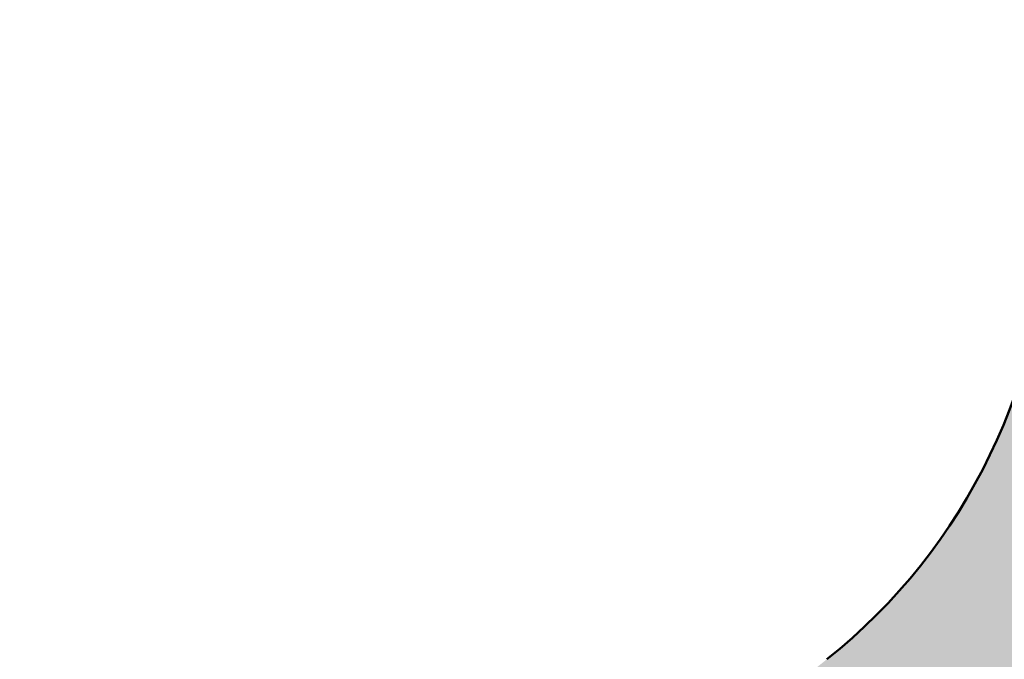
# Model space of a CAD drawing. Units: millimetres. Extents: x 0 to 2267, y 0 to 1823.
# Tile 21 of 256: x 1506 to 1590, y 1162 to 1217. Entities that reach past the tile are written whole.
import ezdxf

# ---------------------------------------------------------------- set-up
doc = ezdxf.new("R2010")
doc.units = ezdxf.units.MM
doc.header["$MEASUREMENT"] = 0
doc.layers.add('M-HATC', color=252, linetype='Continuous', lineweight=18)
doc.layers.add('M-OUTL', color=7, linetype='Continuous', lineweight=50)

msp = doc.modelspace()

# ---------------------------------------------------------------- hatches: boundary and pattern name
at = {"layer": 'M-HATC'}
h = msp.add_hatch(color=256, dxfattribs=at)
h.dxf.hatch_style = 1
h.paths.add_polyline_path([(2055.771, 1603.062), (1381.087, 1603.062), (1381.087, 1598.062), (2055.771, 1598.062)])
h.paths.add_polyline_path([(2055.771, 1598.062), (1381.087, 1598.062), (1381.087, 1593.062), (2055.771, 1593.062)])
h.paths.add_polyline_path([(2051.307, 1536.761), (1385.55, 1536.761), (1385.55, 1526.761), (1387.55, 1526.761), (1388.537, 1525.053), (1385.332, 1521.233), (1385.332, 1521.223), (2050.254, 1522.749), (2048.321, 1525.053), (2049.307, 1526.761), (2051.307, 1526.761)])
edge = h.paths.add_edge_path()
edge.add_arc((1847.535, 1379.149), 135, 222.60306, 222.89085, ccw=False)
edge.add_line((1748.166, 1287.766), (1683.092, 1287.766))
edge.add_arc((1583.724, 1379.149), 135, 317.10915, 317.39694, ccw=False)
edge.add_arc((1678.969, 1290.671), 5, 222.89085, 317.10915, ccw=False)
edge.add_arc((1774.213, 1379.149), 135, 222.60306, 222.89085, ccw=False)
edge.add_line((1674.845, 1287.766), (1609.771, 1287.766))
edge.add_arc((1510.403, 1379.149), 135, 317.10915, 317.39694, ccw=False)
edge.add_arc((1605.647, 1290.671), 5, 222.89085, 317.10915, ccw=False)
edge.add_arc((1700.892, 1379.149), 135, 222.60306, 222.89085, ccw=False)
edge.add_line((1601.524, 1287.766), (1536.45, 1287.766))
edge.add_arc((1437.081, 1379.149), 135, 317.10915, 317.39694, ccw=False)
edge.add_arc((1532.326, 1290.671), 5, 222.89085, 317.10915, ccw=False)
edge.add_arc((1627.571, 1379.149), 135, 222.60306, 222.89085, ccw=False)
edge.add_line((1528.203, 1287.766), (1505.929, 1287.766))
edge.add_spline(control_points=[(1505.929, 1287.766), (1504.262, 1287.766), (1504.262, 1282.766), (1505.929, 1282.766)], knot_values=[0, 0, 0, 0, 5, 5, 5, 5], degree=3, periodic=0)
edge.add_line((1505.929, 1282.766), (1930.929, 1282.766))
edge.add_spline(control_points=[(1930.929, 1282.766), (1932.596, 1282.766), (1932.596, 1287.766), (1930.929, 1287.766)], knot_values=[0, 0, 0, 0, 5, 5, 5, 5], degree=3, periodic=0)
edge.add_line((1930.929, 1287.766), (1903.056, 1287.766))
edge.add_arc((1803.688, 1379.149), 135, 317.10915, 317.39694, ccw=False)
edge.add_arc((1898.932, 1290.671), 5, 222.89085, 317.10915, ccw=False)
edge.add_arc((1994.177, 1379.149), 135, 222.60306, 222.89085, ccw=False)
edge.add_line((1894.809, 1287.766), (1829.735, 1287.766))
edge.add_arc((1730.366, 1379.149), 135, 317.10915, 317.39694, ccw=False)
edge.add_arc((1825.611, 1290.671), 5, 222.89085, 317.10915, ccw=False)
edge.add_arc((1920.856, 1379.149), 135, 222.60306, 222.89085, ccw=False)
edge.add_line((1821.487, 1287.766), (1756.413, 1287.766))
edge.add_arc((1657.045, 1379.149), 135, 317.10915, 317.39694, ccw=False)
edge.add_arc((1752.29, 1290.671), 5, 222.89085, 317.10915, ccw=False)
edge = h.paths.add_edge_path()
edge.add_spline(control_points=[(1843.429, 1227.247), (1845.096, 1227.247), (1845.096, 1232.247), (1843.429, 1232.247)], knot_values=[0, 0, 0, 0, 5, 5, 5, 5], degree=3, periodic=0)
edge.add_line((1843.429, 1232.247), (1593.429, 1232.247))
edge.add_spline(control_points=[(1593.429, 1232.247), (1591.762, 1232.247), (1591.762, 1227.247), (1593.429, 1227.247)], knot_values=[0, 0, 0, 0, 5, 5, 5, 5], degree=3, periodic=0)
edge.add_line((1593.429, 1227.247), (1843.429, 1227.247))
h.paths.add_polyline_path([(1905.929, 1127.417), (1530.929, 1127.417, 0.414214), (1520.929, 1117.417), (1530.929, 1117.417), (1915.929, 1117.417, 0.414214)])
edge = h.paths.add_edge_path()
edge.add_arc((1397.086, 1498.408), 12.73, 90.78215, 190.87871, ccw=False)
edge.add_line((1396.912, 1511.136), (1428.01, 1511.349))
edge.add_line((1428.01, 1511.349), (1433.01, 1511.349))
edge.add_line((1433.01, 1511.349), (1434.439, 1511.349))
edge.add_arc((1419.474, 1498.08), 20, 41.561, 74.08211)
edge.add_line((1424.959, 1517.314), (1399.935, 1517.256))
edge.add_spline(control_points=[(1399.931, 1517.256), (1399.884, 1517.213), (1399.833, 1517.169), (1399.777, 1517.124)], knot_values=[11.567499, 11.567499, 11.567499, 11.567499, 11.814249, 11.814249, 11.814249, 11.814249], degree=3, periodic=0)
edge.add_spline(control_points=[(1399.633, 1517.01), (1399.583, 1516.972), (1399.531, 1516.934), (1399.476, 1516.895)], knot_values=[11.167718, 11.167718, 11.167718, 11.167718, 11.365188, 11.365188, 11.365188, 11.365188], degree=3, periodic=0)
edge.add_spline(control_points=[(1399.34, 1516.8), (1399.151, 1516.672), (1398.938, 1516.538), (1398.704, 1516.399)], knot_values=[10.376405, 10.376405, 10.376405, 10.376405, 11.00994, 11.00994, 11.00994, 11.00994], degree=3, periodic=0)
edge.add_spline(control_points=[(1398.657, 1516.372), (1398.579, 1516.326), (1398.498, 1516.28), (1398.415, 1516.233)], knot_values=[10.125175, 10.125175, 10.125175, 10.125175, 10.334406, 10.334406, 10.334406, 10.334406], degree=3, periodic=0)
edge.add_spline(control_points=[(1398.264, 1516.149), (1398.196, 1516.111), (1398.126, 1516.073), (1398.055, 1516.035)], knot_values=[9.832246, 9.832246, 9.832246, 9.832246, 9.999658, 9.999658, 9.999658, 9.999658], degree=3, periodic=0)
edge.add_spline(control_points=[(1397.999, 1516.005), (1397.731, 1515.862), (1397.446, 1515.717), (1397.147, 1515.571)], knot_values=[9.161808, 9.161808, 9.161808, 9.161808, 9.787769, 9.787769, 9.787769, 9.787769], degree=3, periodic=0)
edge.add_spline(control_points=[(1397.147, 1515.571), (1396.842, 1515.423), (1396.522, 1515.274), (1396.191, 1515.126)], knot_values=[8.524455, 8.524455, 8.524455, 8.524455, 9.161808, 9.161808, 9.161808, 9.161808], degree=3, periodic=0)
edge.add_spline(control_points=[(1396.078, 1515.076), (1395.985, 1515.035), (1395.892, 1514.994), (1395.798, 1514.953)], knot_values=[8.275193, 8.275193, 8.275193, 8.275193, 8.451726, 8.451726, 8.451726, 8.451726], degree=3, periodic=0)
edge.add_spline(control_points=[(1395.602, 1514.869), (1395.5, 1514.826), (1395.397, 1514.782), (1395.293, 1514.739)], knot_values=[7.962917, 7.962917, 7.962917, 7.962917, 8.152764, 8.152764, 8.152764, 8.152764], degree=3, periodic=0)
edge.add_spline(control_points=[(1395.212, 1514.706), (1394.828, 1514.547), (1394.435, 1514.393), (1394.036, 1514.244)], knot_values=[7.21254, 7.21254, 7.21254, 7.21254, 7.913148, 7.913148, 7.913148, 7.913148], degree=3, periodic=0)
edge.add_spline(control_points=[(1394.036, 1514.244), (1393.708, 1514.121), (1393.375, 1514.003), (1393.043, 1513.889)], knot_values=[6.633733, 6.633733, 6.633733, 6.633733, 7.21254, 7.21254, 7.21254, 7.21254], degree=3, periodic=0)
edge.add_spline(control_points=[(1392.821, 1513.815), (1392.72, 1513.781), (1392.618, 1513.748), (1392.517, 1513.715)], knot_values=[6.328796, 6.328796, 6.328796, 6.328796, 6.505493, 6.505493, 6.505493, 6.505493], degree=3, periodic=0)
edge.add_spline(control_points=[(1392.517, 1513.715), (1392.319, 1513.652), (1392.121, 1513.59), (1391.924, 1513.531)], knot_values=[5.984605, 5.984605, 5.984605, 5.984605, 6.328796, 6.328796, 6.328796, 6.328796], degree=3, periodic=0)
edge.add_spline(control_points=[(1391.792, 1513.491), (1391.312, 1513.35), (1390.838, 1513.224), (1390.378, 1513.117)], knot_values=[5.066697, 5.066697, 5.066697, 5.066697, 5.907055, 5.907055, 5.907055, 5.907055], degree=3, periodic=0)
edge.add_spline(control_points=[(1390.378, 1513.117), (1390.18, 1513.071), (1389.984, 1513.028), (1389.791, 1512.99)], knot_values=[4.70367, 4.70367, 4.70367, 4.70367, 5.066695, 5.066695, 5.066695, 5.066695], degree=3, periodic=0)
edge.add_spline(control_points=[(1389.422, 1512.92), (1389.246, 1512.889), (1389.073, 1512.862), (1388.904, 1512.838)], knot_values=[4.130571, 4.130571, 4.130571, 4.130571, 4.469816, 4.469816, 4.469816, 4.469816], degree=3, periodic=0)
edge.add_spline(control_points=[(1388.904, 1512.838), (1388.591, 1512.795), (1388.291, 1512.764), (1388.007, 1512.749)], knot_values=[3.504031, 3.504031, 3.504031, 3.504031, 4.130571, 4.130571, 4.130571, 4.130571], degree=3, periodic=0)
edge.add_spline(control_points=[(1387.936, 1512.746), (1387.854, 1512.742), (1387.773, 1512.74), (1387.694, 1512.739)], knot_values=[3.268866, 3.268866, 3.268866, 3.268866, 3.451164, 3.451164, 3.451164, 3.451164], degree=3, periodic=0)
edge.add_spline(control_points=[(1387.335, 1512.744), (1387.208, 1512.75), (1387.085, 1512.76), (1386.967, 1512.774)], knot_values=[2.670686, 2.670686, 2.670686, 2.670686, 2.984, 2.984, 2.984, 2.984], degree=3, periodic=0)
edge.add_spline(control_points=[(1386.833, 1512.792), (1386.821, 1512.794), (1386.809, 1512.796), (1386.797, 1512.798)], knot_values=[2.516981, 2.516981, 2.516981, 2.516981, 2.549528, 2.549528, 2.549528, 2.549528], degree=3, periodic=0)
edge.add_spline(control_points=[(1386.453, 1512.873), (1386.426, 1512.881), (1386.399, 1512.889), (1386.373, 1512.897)], knot_values=[2.095869, 2.095869, 2.095869, 2.095869, 2.17941, 2.17941, 2.17941, 2.17941], degree=3, periodic=0)
edge.add_spline(control_points=[(1386.069, 1513.019), (1386.063, 1513.022), (1386.058, 1513.025), (1386.052, 1513.028)], knot_values=[1.72453, 1.72453, 1.72453, 1.72453, 1.745933, 1.745933, 1.745933, 1.745933], degree=3, periodic=0)
edge.add_arc((1399.474, 1498.08), 20, 131.82432, 180)
edge.add_arc((1630.334, 1505.548), 250.971, 181.70518, 236.42798)
edge.add_arc((1605.34, 1483.304), 218.782, 238.66083, 243.34961)
edge.add_arc((1647.091, 1510.359), 262.899, 183.12984, 237.85344, ccw=False)
h.paths.add_polyline_path([(1406.537, 1391.964, 0.149382), (1491.551, 1296.442, -0.129517)], flags=17)
edge = h.paths.add_edge_path()
edge.add_arc((2037.384, 1498.08), 20, 0, 48.26587)
edge.add_spline(control_points=[(2050.697, 1513.005), (2050.651, 1512.985), (2050.603, 1512.966), (2050.554, 1512.948)], knot_values=[1.835652, 1.835652, 1.835652, 1.835652, 2.000781, 2.000781, 2.000781, 2.000781], degree=3, periodic=0)
edge.add_spline(control_points=[(2050.462, 1512.917), (2050.479, 1512.922), (2050.496, 1512.928), (2050.513, 1512.934)], knot_values=[2.045477, 2.045477, 2.045477, 2.045477, 2.101389, 2.101389, 2.101389, 2.101389], degree=3, periodic=0)
edge.add_spline(control_points=[(2050.129, 1512.834), (2050.198, 1512.847), (2050.266, 1512.862), (2050.331, 1512.879)], knot_values=[2.237629, 2.237629, 2.237629, 2.237629, 2.435841, 2.435841, 2.435841, 2.435841], degree=3, periodic=0)
edge.add_spline(control_points=[(2050.095, 1512.828), (2050.106, 1512.83), (2050.118, 1512.832), (2050.129, 1512.834)], knot_values=[2.435841, 2.435841, 2.435841, 2.435841, 2.468321, 2.468321, 2.468321, 2.468321], degree=3, periodic=0)
edge.add_spline(control_points=[(2049.784, 1512.785), (2049.855, 1512.792), (2049.924, 1512.801), (2049.992, 1512.811)], knot_values=[2.563852, 2.563852, 2.563852, 2.563852, 2.748541, 2.748541, 2.748541, 2.748541], degree=3, periodic=0)
edge.add_spline(control_points=[(2049.405, 1512.762), (2049.536, 1512.765), (2049.663, 1512.773), (2049.784, 1512.785)], knot_values=[2.748541, 2.748541, 2.748541, 2.748541, 3.064882, 3.064882, 3.064882, 3.064882], degree=3, periodic=0)
edge.add_spline(control_points=[(2049.17, 1512.76), (2049.234, 1512.759), (2049.297, 1512.759), (2049.358, 1512.761)], knot_values=[3.102309, 3.102309, 3.102309, 3.102309, 3.2503, 3.2503, 3.2503, 3.2503], degree=3, periodic=0)
edge.add_spline(control_points=[(2048.857, 1512.769), (2048.964, 1512.764), (2049.068, 1512.761), (2049.17, 1512.76)], knot_values=[3.2503, 3.2503, 3.2503, 3.2503, 3.486069, 3.486069, 3.486069, 3.486069], degree=3, periodic=0)
edge.add_spline(control_points=[(2048.692, 1512.779), (2048.373, 1512.801), (2048.035, 1512.841), (2047.682, 1512.897)], knot_values=[3.606429, 3.606429, 3.606429, 3.606429, 4.2989, 4.2989, 4.2989, 4.2989], degree=3, periodic=0)
edge.add_spline(control_points=[(2047.682, 1512.897), (2047.546, 1512.919), (2047.408, 1512.942), (2047.268, 1512.969)], knot_values=[4.2989, 4.2989, 4.2989, 4.2989, 4.565769, 4.565769, 4.565769, 4.565769], degree=3, periodic=0)
edge.add_spline(control_points=[(2047.268, 1512.969), (2047.145, 1512.991), (2047.021, 1513.016), (2046.895, 1513.042)], knot_values=[4.565769, 4.565769, 4.565769, 4.565769, 4.799971, 4.799971, 4.799971, 4.799971], degree=3, periodic=0)
edge.add_spline(control_points=[(2046.895, 1513.042), (2046.529, 1513.119), (2046.151, 1513.209), (2045.768, 1513.311)], knot_values=[4.799971, 4.799971, 4.799971, 4.799971, 5.483718, 5.483718, 5.483718, 5.483718], degree=3, periodic=0)
edge.add_spline(control_points=[(2045.768, 1513.311), (2045.372, 1513.415), (2044.97, 1513.532), (2044.566, 1513.659)], knot_values=[5.483718, 5.483718, 5.483718, 5.483718, 6.187866, 6.187866, 6.187866, 6.187866], degree=3, periodic=0)
edge.add_spline(control_points=[(2044.566, 1513.659), (2044.415, 1513.706), (2044.263, 1513.755), (2044.112, 1513.805)], knot_values=[6.187866, 6.187866, 6.187866, 6.187866, 6.451551, 6.451551, 6.451551, 6.451551], degree=3, periodic=0)
edge.add_spline(control_points=[(2044.112, 1513.805), (2043.997, 1513.843), (2043.882, 1513.881), (2043.767, 1513.92)], knot_values=[6.451551, 6.451551, 6.451551, 6.451551, 6.651434, 6.651434, 6.651434, 6.651434], degree=3, periodic=0)
edge.add_spline(control_points=[(2043.767, 1513.92), (2043.372, 1514.055), (2042.977, 1514.198), (2042.589, 1514.346)], knot_values=[6.651434, 6.651434, 6.651434, 6.651434, 7.338879, 7.338879, 7.338879, 7.338879], degree=3, periodic=0)
edge.add_spline(control_points=[(2042.589, 1514.346), (2042.164, 1514.507), (2041.746, 1514.675), (2041.341, 1514.846)], knot_values=[7.338879, 7.338879, 7.338879, 7.338879, 8.089209, 8.089209, 8.089209, 8.089209], degree=3, periodic=0)
edge.add_spline(control_points=[(2041.341, 1514.846), (2041.103, 1514.946), (2040.869, 1515.048), (2040.64, 1515.15)], knot_values=[8.089209, 8.089209, 8.089209, 8.089209, 8.529587, 8.529587, 8.529587, 8.529587], degree=3, periodic=0)
edge.add_spline(control_points=[(2040.51, 1515.209), (2040.082, 1515.402), (2039.675, 1515.597), (2039.295, 1515.789)], knot_values=[8.613818, 8.613818, 8.613818, 8.613818, 9.44571, 9.44571, 9.44571, 9.44571], degree=3, periodic=0)
edge.add_spline(control_points=[(2039.295, 1515.789), (2039.062, 1515.907), (2038.839, 1516.025), (2038.629, 1516.14)], knot_values=[9.44571, 9.44571, 9.44571, 9.44571, 9.956404, 9.956404, 9.956404, 9.956404], degree=3, periodic=0)
edge.add_spline(control_points=[(2038.629, 1516.14), (2038.519, 1516.2), (2038.412, 1516.26), (2038.309, 1516.319)], knot_values=[9.956404, 9.956404, 9.956404, 9.956404, 10.223542, 10.223542, 10.223542, 10.223542], degree=3, periodic=0)
edge.add_spline(control_points=[(2038.309, 1516.319), (2038.214, 1516.374), (2038.122, 1516.428), (2038.033, 1516.481)], knot_values=[10.223542, 10.223542, 10.223542, 10.223542, 10.47051, 10.47051, 10.47051, 10.47051], degree=3, periodic=0)
edge.add_spline(control_points=[(2038.033, 1516.481), (2037.786, 1516.63), (2037.564, 1516.773), (2037.372, 1516.909)], knot_values=[10.47051, 10.47051, 10.47051, 10.47051, 11.15767, 11.15767, 11.15767, 11.15767], degree=3, periodic=0)
edge.add_spline(control_points=[(2037.372, 1516.909), (2037.279, 1516.975), (2037.193, 1517.04), (2037.114, 1517.102)], knot_values=[11.15767, 11.15767, 11.15767, 11.15767, 11.49227, 11.49227, 11.49227, 11.49227], degree=3, periodic=0)
edge.add_spline(control_points=[(2036.856, 1517.326), (2036.915, 1517.269), (2036.981, 1517.21), (2037.056, 1517.149)], knot_values=[11.577341, 11.577341, 11.577341, 11.577341, 11.91035, 11.91035, 11.91035, 11.91035], degree=3, periodic=0)
edge.add_spline(control_points=[(2036.807, 1517.375), (2036.823, 1517.359), (2036.839, 1517.342), (2036.856, 1517.326)], knot_values=[11.91035, 11.91035, 11.91035, 11.91035, 12.007402, 12.007402, 12.007402, 12.007402], degree=3, periodic=0)
edge.add_spline(control_points=[(2036.702, 1517.494), (2036.71, 1517.483), (2036.72, 1517.472), (2036.729, 1517.461)], knot_values=[12.184155, 12.184155, 12.184155, 12.184155, 12.255409, 12.255409, 12.255409, 12.255409], degree=3, periodic=0)
edge.add_spline(control_points=[(2036.616, 1517.621), (2036.62, 1517.613), (2036.624, 1517.606), (2036.629, 1517.598)], knot_values=[12.487913, 12.487913, 12.487913, 12.487913, 12.541035, 12.541035, 12.541035, 12.541035], degree=3, periodic=0)
edge.add_spline(control_points=[(2036.563, 1517.786), (2036.564, 1517.779), (2036.564, 1517.773), (2036.565, 1517.766)], knot_values=[12.911761, 12.911761, 12.911761, 12.911761, 12.968286, 12.968286, 12.968286, 12.968286], degree=3, periodic=0)
edge.add_spline(control_points=[(2036.617, 1517.93), (2036.612, 1517.926), (2036.609, 1517.921), (2036.605, 1517.916)], knot_values=[13.382527, 13.382527, 13.382527, 13.382527, 13.433791, 13.433791, 13.433791, 13.433791], degree=3, periodic=0)
edge.add_spline(control_points=[(2036.749, 1518.017), (2036.736, 1518.012), (2036.724, 1518.006), (2036.712, 1518)], knot_values=[13.726299, 13.726299, 13.726299, 13.726299, 13.809928, 13.809928, 13.809928, 13.809928], degree=3, periodic=0)
edge.add_spline(control_points=[(2036.86, 1518.053), (2036.839, 1518.047), (2036.818, 1518.042), (2036.799, 1518.035)], knot_values=[13.910887, 13.910887, 13.910887, 13.910887, 14.02153, 14.02153, 14.02153, 14.02153], degree=3, periodic=0)
edge.add_line((2036.964, 1518.08), (2032.384, 1518.08))
edge.add_line((2032.384, 1518.08), (2027.384, 1518.08))
edge.add_line((2027.384, 1518.08), (2022.384, 1518.08))
edge.add_line((2022.384, 1518.08), (2017.384, 1518.08))
edge.add_arc((2017.384, 1498.08), 20, 90, 138.439)
edge.add_line((2002.419, 1511.349), (2003.848, 1511.349))
edge.add_line((2003.848, 1511.349), (2008.848, 1511.349))
edge.add_line((2008.848, 1511.349), (2039.772, 1511.138))
edge.add_arc((2039.772, 1498.408), 12.73, -10.87871, 90, ccw=False)
edge.add_arc((1789.767, 1510.359), 262.899, 302.14656, 356.87016, ccw=False)
edge.add_arc((1831.518, 1483.304), 218.782, 296.65039, 301.33917)
edge.add_arc((1806.524, 1505.548), 250.971, 303.57202, 358.29482)
h.paths.add_polyline_path([(2030.321, 1391.964, -0.129517), (1945.307, 1296.442, 0.149382)], flags=17)
edge = h.paths.add_edge_path()
edge.add_spline(control_points=[(2037.246, 1518.082), (2037.29, 1518.081), (2037.336, 1518.08), (2037.384, 1518.08)], knot_values=[0.000012, 0.000012, 0.000012, 0.000012, 0.144754, 0.144754, 0.144754, 0.144754], degree=3, periodic=0)
edge.add_line((2037.336, 1518.08), (2037.01, 1518.08))
edge.add_spline(control_points=[(2037.01, 1518.08), (2036.982, 1518.077), (2036.956, 1518.073), (2036.931, 1518.068)], knot_values=[14.13465, 14.13465, 14.13465, 14.13465, 14.247197, 14.247197, 14.247197, 14.247197], degree=3, periodic=0)
edge.add_spline(control_points=[(2036.931, 1518.068), (2036.928, 1518.067), (2036.924, 1518.067), (2036.921, 1518.066)], knot_values=[14.118315, 14.118315, 14.118315, 14.118315, 14.13465, 14.13465, 14.13465, 14.13465], degree=3, periodic=0)
edge.add_spline(control_points=[(2036.921, 1518.066), (2036.912, 1518.064), (2036.903, 1518.063), (2036.895, 1518.061)], knot_values=[14.078086, 14.078086, 14.078086, 14.078086, 14.118315, 14.118315, 14.118315, 14.118315], degree=3, periodic=0)
edge.add_spline(control_points=[(2036.895, 1518.061), (2036.883, 1518.058), (2036.872, 1518.056), (2036.86, 1518.053)], knot_values=[14.02153, 14.02153, 14.02153, 14.02153, 14.078086, 14.078086, 14.078086, 14.078086], degree=3, periodic=0)
edge.add_spline(control_points=[(2036.86, 1518.053), (2036.839, 1518.047), (2036.818, 1518.042), (2036.799, 1518.035)], knot_values=[13.910887, 13.910887, 13.910887, 13.910887, 14.02153, 14.02153, 14.02153, 14.02153], degree=3, periodic=0)
edge.add_spline(control_points=[(2036.799, 1518.035), (2036.798, 1518.035), (2036.797, 1518.035), (2036.797, 1518.035)], knot_values=[13.906906, 13.906906, 13.906906, 13.906906, 13.910887, 13.910887, 13.910887, 13.910887], degree=3, periodic=0)
edge.add_spline(control_points=[(2036.797, 1518.035), (2036.788, 1518.032), (2036.78, 1518.029), (2036.772, 1518.026)], knot_values=[13.857826, 13.857826, 13.857826, 13.857826, 13.906906, 13.906906, 13.906906, 13.906906], degree=3, periodic=0)
edge.add_spline(control_points=[(2036.772, 1518.026), (2036.764, 1518.023), (2036.756, 1518.02), (2036.749, 1518.017)], knot_values=[13.809928, 13.809928, 13.809928, 13.809928, 13.857826, 13.857826, 13.857826, 13.857826], degree=3, periodic=0)
edge.add_spline(control_points=[(2036.749, 1518.017), (2036.736, 1518.012), (2036.724, 1518.006), (2036.712, 1518)], knot_values=[13.726299, 13.726299, 13.726299, 13.726299, 13.809928, 13.809928, 13.809928, 13.809928], degree=3, periodic=0)
edge.add_spline(control_points=[(2036.712, 1518), (2036.712, 1518), (2036.712, 1518), (2036.711, 1518)], knot_values=[13.723993, 13.723993, 13.723993, 13.723993, 13.726299, 13.726299, 13.726299, 13.726299], degree=3, periodic=0)
edge.add_spline(control_points=[(2036.711, 1518), (2036.706, 1517.997), (2036.701, 1517.994), (2036.696, 1517.992)], knot_values=[13.686536, 13.686536, 13.686536, 13.686536, 13.723993, 13.723993, 13.723993, 13.723993], degree=3, periodic=0)
edge.add_spline(control_points=[(2036.696, 1517.992), (2036.692, 1517.989), (2036.687, 1517.987), (2036.683, 1517.984)], knot_values=[13.651251, 13.651251, 13.651251, 13.651251, 13.686536, 13.686536, 13.686536, 13.686536], degree=3, periodic=0)
edge.add_spline(control_points=[(2036.683, 1517.984), (2036.676, 1517.98), (2036.67, 1517.976), (2036.664, 1517.971)], knot_values=[13.596804, 13.596804, 13.596804, 13.596804, 13.651251, 13.651251, 13.651251, 13.651251], degree=3, periodic=0)
edge.add_spline(control_points=[(2036.664, 1517.971), (2036.664, 1517.971), (2036.663, 1517.971), (2036.663, 1517.971)], knot_values=[13.593956, 13.593956, 13.593956, 13.593956, 13.596804, 13.596804, 13.596804, 13.596804], degree=3, periodic=0)
edge.add_spline(control_points=[(2036.663, 1517.971), (2036.66, 1517.969), (2036.658, 1517.967), (2036.655, 1517.965)], knot_values=[13.570322, 13.570322, 13.570322, 13.570322, 13.593956, 13.593956, 13.593956, 13.593956], degree=3, periodic=0)
edge.add_spline(control_points=[(2036.655, 1517.965), (2036.653, 1517.963), (2036.65, 1517.961), (2036.647, 1517.959)], knot_values=[13.545477, 13.545477, 13.545477, 13.545477, 13.570322, 13.570322, 13.570322, 13.570322], degree=3, periodic=0)
edge.add_spline(control_points=[(2036.647, 1517.959), (2036.647, 1517.959), (2036.647, 1517.959), (2036.647, 1517.959)], knot_values=[13.543931, 13.543931, 13.543931, 13.543931, 13.545477, 13.545477, 13.545477, 13.545477], degree=3, periodic=0)
edge.add_spline(control_points=[(2036.647, 1517.959), (2036.641, 1517.954), (2036.636, 1517.949), (2036.631, 1517.945)], knot_values=[13.488237, 13.488237, 13.488237, 13.488237, 13.543931, 13.543931, 13.543931, 13.543931], degree=3, periodic=0)
edge.add_spline(control_points=[(2036.631, 1517.945), (2036.628, 1517.942), (2036.626, 1517.94), (2036.623, 1517.937)], knot_values=[13.460307, 13.460307, 13.460307, 13.460307, 13.488237, 13.488237, 13.488237, 13.488237], degree=3, periodic=0)
edge.add_spline(control_points=[(2036.623, 1517.937), (2036.622, 1517.936), (2036.62, 1517.934), (2036.618, 1517.932)], knot_values=[13.439712, 13.439712, 13.439712, 13.439712, 13.460307, 13.460307, 13.460307, 13.460307], degree=3, periodic=0)
edge.add_spline(control_points=[(2036.618, 1517.932), (2036.618, 1517.931), (2036.617, 1517.931), (2036.617, 1517.93)], knot_values=[13.433791, 13.433791, 13.433791, 13.433791, 13.439712, 13.439712, 13.439712, 13.439712], degree=3, periodic=0)
edge.add_spline(control_points=[(2036.617, 1517.93), (2036.612, 1517.926), (2036.609, 1517.921), (2036.605, 1517.916)], knot_values=[13.382527, 13.382527, 13.382527, 13.382527, 13.433791, 13.433791, 13.433791, 13.433791], degree=3, periodic=0)
edge.add_spline(control_points=[(2036.605, 1517.916), (2036.603, 1517.913), (2036.6, 1517.91), (2036.598, 1517.907)], knot_values=[13.350017, 13.350017, 13.350017, 13.350017, 13.382527, 13.382527, 13.382527, 13.382527], degree=3, periodic=0)
edge.add_spline(control_points=[(2036.598, 1517.907), (2036.597, 1517.906), (2036.596, 1517.904), (2036.595, 1517.903)], knot_values=[13.333922, 13.333922, 13.333922, 13.333922, 13.350017, 13.350017, 13.350017, 13.350017], degree=3, periodic=0)
edge.add_spline(control_points=[(2036.595, 1517.903), (2036.595, 1517.902), (2036.594, 1517.901), (2036.593, 1517.9)], knot_values=[13.323828, 13.323828, 13.323828, 13.323828, 13.333922, 13.333922, 13.333922, 13.333922], degree=3, periodic=0)
edge.add_spline(control_points=[(2036.593, 1517.9), (2036.59, 1517.895), (2036.588, 1517.891), (2036.585, 1517.886)], knot_values=[13.277545, 13.277545, 13.277545, 13.277545, 13.323828, 13.323828, 13.323828, 13.323828], degree=3, periodic=0)
edge.add_spline(control_points=[(2036.585, 1517.886), (2036.584, 1517.883), (2036.582, 1517.879), (2036.58, 1517.875)], knot_values=[13.240119, 13.240119, 13.240119, 13.240119, 13.277545, 13.277545, 13.277545, 13.277545], degree=3, periodic=0)
edge.add_spline(control_points=[(2036.58, 1517.875), (2036.58, 1517.874), (2036.579, 1517.873), (2036.578, 1517.872)], knot_values=[13.228211, 13.228211, 13.228211, 13.228211, 13.240119, 13.240119, 13.240119, 13.240119], degree=3, periodic=0)
edge.add_spline(control_points=[(2036.578, 1517.872), (2036.578, 1517.87), (2036.577, 1517.869), (2036.577, 1517.868)], knot_values=[13.215717, 13.215717, 13.215717, 13.215717, 13.228211, 13.228211, 13.228211, 13.228211], degree=3, periodic=0)
edge.add_spline(control_points=[(2036.577, 1517.868), (2036.575, 1517.864), (2036.574, 1517.86), (2036.573, 1517.857)], knot_values=[13.179847, 13.179847, 13.179847, 13.179847, 13.215717, 13.215717, 13.215717, 13.215717], degree=3, periodic=0)
edge.add_spline(control_points=[(2036.573, 1517.857), (2036.571, 1517.851), (2036.57, 1517.846), (2036.569, 1517.841)], knot_values=[13.132017, 13.132017, 13.132017, 13.132017, 13.179847, 13.179847, 13.179847, 13.179847], degree=3, periodic=0)
edge.add_spline(control_points=[(2036.569, 1517.841), (2036.568, 1517.84), (2036.568, 1517.839), (2036.568, 1517.838)], knot_values=[13.122482, 13.122482, 13.122482, 13.122482, 13.132017, 13.132017, 13.132017, 13.132017], degree=3, periodic=0)
edge.add_spline(control_points=[(2036.568, 1517.838), (2036.568, 1517.836), (2036.567, 1517.835), (2036.567, 1517.833)], knot_values=[13.105592, 13.105592, 13.105592, 13.105592, 13.122482, 13.122482, 13.122482, 13.122482], degree=3, periodic=0)
edge.add_spline(control_points=[(2036.567, 1517.833), (2036.566, 1517.829), (2036.566, 1517.826), (2036.565, 1517.822)], knot_values=[13.074063, 13.074063, 13.074063, 13.074063, 13.105592, 13.105592, 13.105592, 13.105592], degree=3, periodic=0)
edge.add_spline(control_points=[(2036.565, 1517.822), (2036.565, 1517.822), (2036.565, 1517.822), (2036.565, 1517.822)], knot_values=[13.074043, 13.074043, 13.074043, 13.074043, 13.074063, 13.074063, 13.074063, 13.074063], degree=3, periodic=0)
edge.add_spline(control_points=[(2036.565, 1517.822), (2036.564, 1517.816), (2036.564, 1517.811), (2036.564, 1517.805)], knot_values=[13.021884, 13.021884, 13.021884, 13.021884, 13.074043, 13.074043, 13.074043, 13.074043], degree=3, periodic=0)
edge.add_spline(control_points=[(2036.564, 1517.805), (2036.564, 1517.804), (2036.564, 1517.803), (2036.564, 1517.803)], knot_values=[13.01674, 13.01674, 13.01674, 13.01674, 13.021884, 13.021884, 13.021884, 13.021884], degree=3, periodic=0)
edge.add_spline(control_points=[(2036.564, 1517.803), (2036.563, 1517.801), (2036.563, 1517.798), (2036.563, 1517.796)], knot_values=[12.996438, 12.996438, 12.996438, 12.996438, 13.01674, 13.01674, 13.01674, 13.01674], degree=3, periodic=0)
edge.add_spline(control_points=[(2036.563, 1517.796), (2036.563, 1517.793), (2036.563, 1517.789), (2036.563, 1517.786)], knot_values=[12.968286, 12.968286, 12.968286, 12.968286, 12.996438, 12.996438, 12.996438, 12.996438], degree=3, periodic=0)
edge.add_spline(control_points=[(2036.563, 1517.786), (2036.564, 1517.779), (2036.564, 1517.773), (2036.565, 1517.766)], knot_values=[12.911761, 12.911761, 12.911761, 12.911761, 12.968286, 12.968286, 12.968286, 12.968286], degree=3, periodic=0)
edge.add_spline(control_points=[(2036.565, 1517.766), (2036.565, 1517.766), (2036.565, 1517.766), (2036.565, 1517.766)], knot_values=[12.911017, 12.911017, 12.911017, 12.911017, 12.911761, 12.911761, 12.911761, 12.911761], degree=3, periodic=0)
edge.add_spline(control_points=[(2036.565, 1517.766), (2036.565, 1517.762), (2036.566, 1517.759), (2036.566, 1517.756)], knot_values=[12.88528, 12.88528, 12.88528, 12.88528, 12.911017, 12.911017, 12.911017, 12.911017], degree=3, periodic=0)
edge.add_spline(control_points=[(2036.566, 1517.756), (2036.567, 1517.753), (2036.567, 1517.751), (2036.568, 1517.748)], knot_values=[12.862519, 12.862519, 12.862519, 12.862519, 12.88528, 12.88528, 12.88528, 12.88528], degree=3, periodic=0)
edge.add_spline(control_points=[(2036.568, 1517.748), (2036.568, 1517.747), (2036.568, 1517.747), (2036.568, 1517.746)], knot_values=[12.858885, 12.858885, 12.858885, 12.858885, 12.862519, 12.862519, 12.862519, 12.862519], degree=3, periodic=0)
edge.add_spline(control_points=[(2036.568, 1517.746), (2036.569, 1517.74), (2036.571, 1517.733), (2036.572, 1517.726)], knot_values=[12.8053, 12.8053, 12.8053, 12.8053, 12.858885, 12.858885, 12.858885, 12.858885], degree=3, periodic=0)
edge.add_spline(control_points=[(2036.572, 1517.726), (2036.573, 1517.723), (2036.574, 1517.719), (2036.576, 1517.715)], knot_values=[12.775176, 12.775176, 12.775176, 12.775176, 12.8053, 12.8053, 12.8053, 12.8053], degree=3, periodic=0)
edge.add_spline(control_points=[(2036.576, 1517.715), (2036.576, 1517.713), (2036.577, 1517.71), (2036.578, 1517.708)], knot_values=[12.756759, 12.756759, 12.756759, 12.756759, 12.775176, 12.775176, 12.775176, 12.775176], degree=3, periodic=0)
edge.add_spline(control_points=[(2036.578, 1517.708), (2036.578, 1517.707), (2036.578, 1517.706), (2036.579, 1517.705)], knot_values=[12.748742, 12.748742, 12.748742, 12.748742, 12.756759, 12.756759, 12.756759, 12.756759], degree=3, periodic=0)
edge.add_spline(control_points=[(2036.579, 1517.705), (2036.581, 1517.698), (2036.583, 1517.692), (2036.586, 1517.685)], knot_values=[12.69959, 12.69959, 12.69959, 12.69959, 12.748742, 12.748742, 12.748742, 12.748742], degree=3, periodic=0)
edge.add_spline(control_points=[(2036.586, 1517.685), (2036.588, 1517.68), (2036.59, 1517.675), (2036.592, 1517.669)], knot_values=[12.659038, 12.659038, 12.659038, 12.659038, 12.69959, 12.69959, 12.69959, 12.69959], degree=3, periodic=0)
edge.add_spline(control_points=[(2036.592, 1517.669), (2036.594, 1517.665), (2036.596, 1517.66), (2036.598, 1517.656)], knot_values=[12.626806, 12.626806, 12.626806, 12.626806, 12.659038, 12.659038, 12.659038, 12.659038], degree=3, periodic=0)
edge.add_spline(control_points=[(2036.598, 1517.656), (2036.598, 1517.655), (2036.599, 1517.654), (2036.599, 1517.653)], knot_values=[12.619394, 12.619394, 12.619394, 12.619394, 12.626806, 12.626806, 12.626806, 12.626806], degree=3, periodic=0)
edge.add_spline(control_points=[(2036.599, 1517.653), (2036.604, 1517.642), (2036.61, 1517.632), (2036.616, 1517.621)], knot_values=[12.541039, 12.541039, 12.541039, 12.541039, 12.619394, 12.619394, 12.619394, 12.619394], degree=3, periodic=0)
edge.add_spline(control_points=[(2036.616, 1517.621), (2036.616, 1517.621), (2036.616, 1517.621), (2036.616, 1517.621)], knot_values=[12.541035, 12.541035, 12.541035, 12.541035, 12.541039, 12.541039, 12.541039, 12.541039], degree=3, periodic=0)
edge.add_spline(control_points=[(2036.616, 1517.621), (2036.62, 1517.613), (2036.624, 1517.606), (2036.629, 1517.598)], knot_values=[12.487913, 12.487913, 12.487913, 12.487913, 12.541035, 12.541035, 12.541035, 12.541035], degree=3, periodic=0)
edge.add_spline(control_points=[(2036.629, 1517.598), (2036.633, 1517.592), (2036.637, 1517.585), (2036.641, 1517.579)], knot_values=[12.443982, 12.443982, 12.443982, 12.443982, 12.487913, 12.487913, 12.487913, 12.487913], degree=3, periodic=0)
edge.add_spline(control_points=[(2036.641, 1517.579), (2036.641, 1517.578), (2036.642, 1517.576), (2036.643, 1517.575)], knot_values=[12.434996, 12.434996, 12.434996, 12.434996, 12.443982, 12.443982, 12.443982, 12.443982], degree=3, periodic=0)
edge.add_spline(control_points=[(2036.643, 1517.575), (2036.653, 1517.56), (2036.664, 1517.544), (2036.676, 1517.528)], knot_values=[12.329647, 12.329647, 12.329647, 12.329647, 12.434996, 12.434996, 12.434996, 12.434996], degree=3, periodic=0)
edge.add_spline(control_points=[(2036.676, 1517.528), (2036.684, 1517.517), (2036.693, 1517.505), (2036.702, 1517.494)], knot_values=[12.255409, 12.255409, 12.255409, 12.255409, 12.329647, 12.329647, 12.329647, 12.329647], degree=3, periodic=0)
edge.add_spline(control_points=[(2036.702, 1517.494), (2036.71, 1517.483), (2036.72, 1517.472), (2036.729, 1517.461)], knot_values=[12.184155, 12.184155, 12.184155, 12.184155, 12.255409, 12.255409, 12.255409, 12.255409], degree=3, periodic=0)
edge.add_spline(control_points=[(2036.729, 1517.461), (2036.744, 1517.444), (2036.759, 1517.426), (2036.775, 1517.409)], knot_values=[12.075961, 12.075961, 12.075961, 12.075961, 12.184155, 12.184155, 12.184155, 12.184155], degree=3, periodic=0)
edge.add_spline(control_points=[(2036.775, 1517.409), (2036.776, 1517.407), (2036.777, 1517.406), (2036.778, 1517.405)], knot_values=[12.069502, 12.069502, 12.069502, 12.069502, 12.075961, 12.075961, 12.075961, 12.075961], degree=3, periodic=0)
edge.add_spline(control_points=[(2036.778, 1517.405), (2036.788, 1517.395), (2036.797, 1517.385), (2036.807, 1517.375)], knot_values=[12.007402, 12.007402, 12.007402, 12.007402, 12.069502, 12.069502, 12.069502, 12.069502], degree=3, periodic=0)
edge.add_spline(control_points=[(2036.807, 1517.375), (2036.823, 1517.359), (2036.839, 1517.342), (2036.856, 1517.326)], knot_values=[11.91035, 11.91035, 11.91035, 11.91035, 12.007402, 12.007402, 12.007402, 12.007402], degree=3, periodic=0)
edge.add_spline(control_points=[(2036.856, 1517.326), (2036.915, 1517.269), (2036.981, 1517.21), (2037.056, 1517.149)], knot_values=[11.577341, 11.577341, 11.577341, 11.577341, 11.91035, 11.91035, 11.91035, 11.91035], degree=3, periodic=0)
edge.add_spline(control_points=[(2037.056, 1517.149), (2037.075, 1517.134), (2037.094, 1517.118), (2037.114, 1517.102)], knot_values=[11.49227, 11.49227, 11.49227, 11.49227, 11.577341, 11.577341, 11.577341, 11.577341], degree=3, periodic=0)
edge.add_spline(control_points=[(2037.114, 1517.102), (2037.193, 1517.04), (2037.279, 1516.975), (2037.372, 1516.909)], knot_values=[11.15767, 11.15767, 11.15767, 11.15767, 11.49227, 11.49227, 11.49227, 11.49227], degree=3, periodic=0)
edge.add_spline(control_points=[(2037.372, 1516.909), (2037.564, 1516.773), (2037.786, 1516.63), (2038.033, 1516.481)], knot_values=[10.47051, 10.47051, 10.47051, 10.47051, 11.15767, 11.15767, 11.15767, 11.15767], degree=3, periodic=0)
edge.add_spline(control_points=[(2038.033, 1516.481), (2038.122, 1516.428), (2038.214, 1516.374), (2038.309, 1516.319)], knot_values=[10.223542, 10.223542, 10.223542, 10.223542, 10.47051, 10.47051, 10.47051, 10.47051], degree=3, periodic=0)
edge.add_spline(control_points=[(2038.309, 1516.319), (2038.412, 1516.26), (2038.519, 1516.2), (2038.629, 1516.14)], knot_values=[9.956404, 9.956404, 9.956404, 9.956404, 10.223542, 10.223542, 10.223542, 10.223542], degree=3, periodic=0)
edge.add_spline(control_points=[(2038.629, 1516.14), (2038.839, 1516.025), (2039.062, 1515.907), (2039.295, 1515.789)], knot_values=[9.44571, 9.44571, 9.44571, 9.44571, 9.956404, 9.956404, 9.956404, 9.956404], degree=3, periodic=0)
edge.add_spline(control_points=[(2039.295, 1515.789), (2039.675, 1515.597), (2040.082, 1515.402), (2040.51, 1515.209)], knot_values=[8.613818, 8.613818, 8.613818, 8.613818, 9.44571, 9.44571, 9.44571, 9.44571], degree=3, periodic=0)
edge.add_spline(control_points=[(2040.51, 1515.209), (2040.553, 1515.189), (2040.597, 1515.17), (2040.64, 1515.15)], knot_values=[8.529587, 8.529587, 8.529587, 8.529587, 8.613818, 8.613818, 8.613818, 8.613818], degree=3, periodic=0)
edge.add_spline(control_points=[(2040.64, 1515.15), (2040.869, 1515.048), (2041.103, 1514.946), (2041.341, 1514.846)], knot_values=[8.089209, 8.089209, 8.089209, 8.089209, 8.529587, 8.529587, 8.529587, 8.529587], degree=3, periodic=0)
edge.add_spline(control_points=[(2041.341, 1514.846), (2041.746, 1514.675), (2042.164, 1514.507), (2042.589, 1514.346)], knot_values=[7.338879, 7.338879, 7.338879, 7.338879, 8.089209, 8.089209, 8.089209, 8.089209], degree=3, periodic=0)
edge.add_spline(control_points=[(2042.589, 1514.346), (2042.977, 1514.198), (2043.372, 1514.055), (2043.767, 1513.92)], knot_values=[6.651434, 6.651434, 6.651434, 6.651434, 7.338879, 7.338879, 7.338879, 7.338879], degree=3, periodic=0)
edge.add_spline(control_points=[(2043.767, 1513.92), (2043.882, 1513.881), (2043.997, 1513.843), (2044.112, 1513.805)], knot_values=[6.451551, 6.451551, 6.451551, 6.451551, 6.651434, 6.651434, 6.651434, 6.651434], degree=3, periodic=0)
edge.add_spline(control_points=[(2044.112, 1513.805), (2044.263, 1513.755), (2044.415, 1513.706), (2044.566, 1513.659)], knot_values=[6.187866, 6.187866, 6.187866, 6.187866, 6.451551, 6.451551, 6.451551, 6.451551], degree=3, periodic=0)
edge.add_spline(control_points=[(2044.566, 1513.659), (2044.97, 1513.532), (2045.372, 1513.415), (2045.768, 1513.311)], knot_values=[5.483718, 5.483718, 5.483718, 5.483718, 6.187866, 6.187866, 6.187866, 6.187866], degree=3, periodic=0)
edge.add_spline(control_points=[(2045.768, 1513.311), (2046.151, 1513.209), (2046.529, 1513.119), (2046.895, 1513.042)], knot_values=[4.799971, 4.799971, 4.799971, 4.799971, 5.483718, 5.483718, 5.483718, 5.483718], degree=3, periodic=0)
edge.add_spline(control_points=[(2046.895, 1513.042), (2047.021, 1513.016), (2047.145, 1512.991), (2047.268, 1512.969)], knot_values=[4.565769, 4.565769, 4.565769, 4.565769, 4.799971, 4.799971, 4.799971, 4.799971], degree=3, periodic=0)
edge.add_spline(control_points=[(2047.268, 1512.969), (2047.408, 1512.942), (2047.546, 1512.919), (2047.682, 1512.897)], knot_values=[4.2989, 4.2989, 4.2989, 4.2989, 4.565769, 4.565769, 4.565769, 4.565769], degree=3, periodic=0)
edge.add_spline(control_points=[(2047.682, 1512.897), (2048.035, 1512.841), (2048.373, 1512.801), (2048.692, 1512.779)], knot_values=[3.606429, 3.606429, 3.606429, 3.606429, 4.2989, 4.2989, 4.2989, 4.2989], degree=3, periodic=0)
edge.add_spline(control_points=[(2048.692, 1512.779), (2048.748, 1512.775), (2048.803, 1512.772), (2048.857, 1512.769)], knot_values=[3.486069, 3.486069, 3.486069, 3.486069, 3.606429, 3.606429, 3.606429, 3.606429], degree=3, periodic=0)
edge.add_spline(control_points=[(2048.857, 1512.769), (2048.964, 1512.764), (2049.068, 1512.761), (2049.17, 1512.76)], knot_values=[3.2503, 3.2503, 3.2503, 3.2503, 3.486069, 3.486069, 3.486069, 3.486069], degree=3, periodic=0)
edge.add_spline(control_points=[(2049.17, 1512.76), (2049.234, 1512.759), (2049.297, 1512.759), (2049.358, 1512.761)], knot_values=[3.102309, 3.102309, 3.102309, 3.102309, 3.2503, 3.2503, 3.2503, 3.2503], degree=3, periodic=0)
edge.add_spline(control_points=[(2049.358, 1512.761), (2049.374, 1512.761), (2049.39, 1512.761), (2049.405, 1512.762)], knot_values=[3.064882, 3.064882, 3.064882, 3.064882, 3.102309, 3.102309, 3.102309, 3.102309], degree=3, periodic=0)
edge.add_spline(control_points=[(2049.405, 1512.762), (2049.536, 1512.765), (2049.663, 1512.773), (2049.784, 1512.785)], knot_values=[2.748541, 2.748541, 2.748541, 2.748541, 3.064882, 3.064882, 3.064882, 3.064882], degree=3, periodic=0)
edge.add_spline(control_points=[(2049.784, 1512.785), (2049.855, 1512.792), (2049.924, 1512.801), (2049.992, 1512.811)], knot_values=[2.563852, 2.563852, 2.563852, 2.563852, 2.748541, 2.748541, 2.748541, 2.748541], degree=3, periodic=0)
edge.add_spline(control_points=[(2049.992, 1512.811), (2050.026, 1512.816), (2050.061, 1512.822), (2050.095, 1512.828)], knot_values=[2.468321, 2.468321, 2.468321, 2.468321, 2.563852, 2.563852, 2.563852, 2.563852], degree=3, periodic=0)
edge.add_spline(control_points=[(2050.095, 1512.828), (2050.106, 1512.83), (2050.118, 1512.832), (2050.129, 1512.834)], knot_values=[2.435841, 2.435841, 2.435841, 2.435841, 2.468321, 2.468321, 2.468321, 2.468321], degree=3, periodic=0)
edge.add_spline(control_points=[(2050.129, 1512.834), (2050.198, 1512.847), (2050.266, 1512.862), (2050.331, 1512.879)], knot_values=[2.237629, 2.237629, 2.237629, 2.237629, 2.435841, 2.435841, 2.435841, 2.435841], degree=3, periodic=0)
edge.add_spline(control_points=[(2050.331, 1512.879), (2050.375, 1512.891), (2050.419, 1512.903), (2050.462, 1512.917)], knot_values=[2.101389, 2.101389, 2.101389, 2.101389, 2.237629, 2.237629, 2.237629, 2.237629], degree=3, periodic=0)
edge.add_spline(control_points=[(2050.462, 1512.917), (2050.479, 1512.922), (2050.496, 1512.928), (2050.513, 1512.934)], knot_values=[2.045477, 2.045477, 2.045477, 2.045477, 2.101389, 2.101389, 2.101389, 2.101389], degree=3, periodic=0)
edge.add_spline(control_points=[(2050.513, 1512.934), (2050.527, 1512.938), (2050.54, 1512.943), (2050.554, 1512.948)], knot_values=[2.000781, 2.000781, 2.000781, 2.000781, 2.045477, 2.045477, 2.045477, 2.045477], degree=3, periodic=0)
edge.add_spline(control_points=[(2050.554, 1512.948), (2050.603, 1512.966), (2050.651, 1512.985), (2050.697, 1513.005)], knot_values=[1.835652, 1.835652, 1.835652, 1.835652, 2.000781, 2.000781, 2.000781, 2.000781], degree=3, periodic=0)
edge.add_arc((2037.384, 1498.08), 20, 48.26587, 90.12993)
edge = h.paths.add_edge_path(flags=16)
edge.add_spline(control_points=[(1386.139, 1512.986), (1388.92, 1511.739), (1398.039, 1515.519), (1399.931, 1517.256)], knot_values=[1.831046, 1.831046, 1.831046, 1.831046, 11.814249, 11.814249, 11.814249, 11.814249], degree=3, periodic=0)
edge.add_line((1399.931, 1517.256), (1393.743, 1517.242))
edge.add_arc((1399.474, 1498.08), 20, 106.6501, 131.8173)
h = msp.add_hatch(color=256, dxfattribs=at)
h.dxf.hatch_style = 1
h.paths.add_polyline_path([(2042.889, 1580.18), (2055.771, 1593.062), (1381.087, 1593.062), (1393.969, 1580.18), (1374.086, 1560.296), (2062.772, 1560.296)])
h.paths.add_polyline_path([(1843.429, 1201.33), (1843.429, 1227.247), (1593.429, 1227.247), (1593.429, 1201.33, -0.228274), (1574.599, 1162.235), (1530.929, 1127.417), (1905.929, 1127.417), (1862.259, 1162.235, -0.228274)])

# ---------------------------------------------------------------- linework, layer by layer
at = {"layer": 'M-OUTL'}
msp.add_arc((1543.429, 1201.33), 50, 308.56488, 0, dxfattribs=at)

doc.saveas('drawing.dxf')
